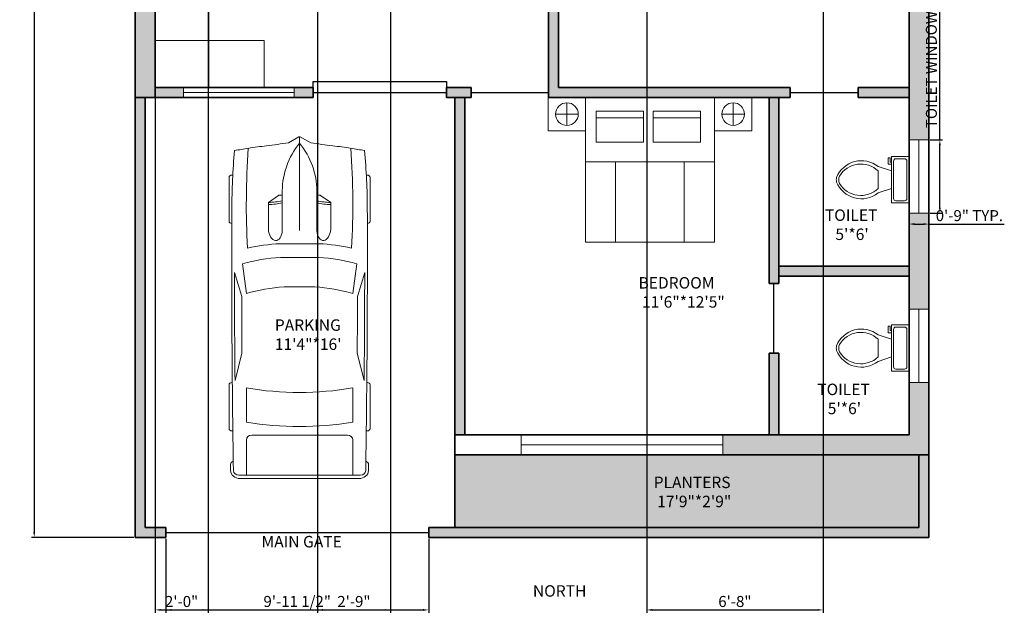
# Model space of a CAD drawing. Units: inches. Extents: x 2066 to 2563, y 1438 to 2142.
# Tile 1 of 3: x 2066 to 2512, y 1438 to 1710. Entities that reach past the tile are written whole.
import ezdxf

# ---------------------------------------------------------------- set-up
doc = ezdxf.new("R2010")
doc.units = ezdxf.units.IN
for name, color, linetype, lineweight in [('A-ANNO-DIMS', 2, 'Continuous', 18), ('A-ANNO-TEXT', 10, 'Continuous', 18), ('A-AREA-IDEN', 10, 'Continuous', 18), ('A-DOOR', 4, 'Continuous', 25), ('A-FLOR-FIXT', 8, 'Continuous', 18), ('A-SITE-VEHS', 8, 'Continuous', 13), ('A-WALL-PATT', 140, 'Continuous', 13), ('BED', 31, 'Continuous', 18), ('FUR', 191, 'Continuous', 18), ('L-PLNT-PATT', 84, 'Continuous', 13), ('WALL', 7, 'Continuous', 35), ('WIND', 210, 'Continuous', 18)]:
    doc.layers.add(name, color=color, linetype=linetype, lineweight=lineweight)
doc.styles.get("Standard").update_dxf_attribs({"font": 'arial.ttf'})
doc.dimstyles.new('ISO-25', dxfattribs={"dimtxt": 5, "dimasz": 2.5, "dimexe": 1.25, "dimexo": 0.625, "dimtad": 1, "dimdec": 0, "dimlunit": 4, "dimtxsty": 'Standard', "dimcen": 2.5, "dimadec": 0, "dimazin": 0, "dimtfac": 1, "dimtdec": 0, "dimtmove": 0, "dimatfit": 3, "dimfxl": 1, "dimarcsym": 0})

# ---------------------------------------------------------------- blocks, each defined once
blk = doc.blocks.new('*U3')
for p, q in [((9.5, -6), (9.5, -2)), ((-10, -8.5), (-8, -8.5)), ((-10, -9.5), (-10, -8.5)), ((-8, -8.5), (-8, -8)), ((-7, -8), (-7, -9.5)), ((-4, -8), (-6, -14)), ((4, -8), (6, -14)), ((-7, -9.5), (-10, -9.5)), ((4, -14), (-4, -14))]:
    blk.add_line(p, q)
blk.add_lwpolyline([(10.5, -8), (10.5, 0), (-10.5, 0), (-10.5, -8)], close=True)
for points in [[(-9.5, -2), (-9.5, -6)], [(8.5, -1), (-8.5, -1)], [(-8.5, -7), (8.5, -7)]]:
    blk.add_lwpolyline(points)
for centre, radius, start, end in [((-8.62, -1.88), 0.884, 81.8699, 188.1301), ((8.62, -1.88), 0.884, 351.8699, 98.1301), ((-8.62, -6.12), 0.884, 171.8699, 278.1301), ((8.62, -6.12), 0.884, 261.8699, 8.1301), ((3.52, -21.58), 12.17, 141.4691, 247.9714), ((4.2, -21.82), 11.33, 136.3677, 238.9468), ((-3.52, -21.58), 12.17, 292.0284, 38.5307), ((-4.2, -21.82), 11.33, 301.053, 43.6321), ((0, -27.88), 4, 245.7318, 294.2682), ((0, -29), 4, 254.8605, 285.1395)]:
    blk.add_arc(centre, radius, start, end)
blk = doc.blocks.new('*U5')
for p, q in [((46.55, 38.89), (22.35, 38.89)), ((136.7, 38.89), (160.9, 38.89)), ((21.1, 37.41), (21.1, 36.83)), ((47.8, 37.39), (47.8, 37.41)), ((87.99, 31.87), (74.76, 35.92)), ((134.31, 35.6), (119.29, 31.78)), ((135.45, 37.07), (135.45, 37.41)), ((162.15, 37.41), (162.15, 36.77)), ((186.47, -33.5), (186.47, 33.5)), ((188.4, -32.76), (188.4, 32.76)), ((70.03, 31.54), (86.41, 29.35)), ((138.42, 29.35), (157.25, 29.35)), ((186.47, 29.35), (167.01, 29.35)), ((164.52, 26.39), (164.52, -26.39)), ((32.27, 11.63), (36.13, 17.17)), ((36.13, 17.17), (50.94, 17.17)), ((32.12, 9.51), (32.12, 11.15)), ((3.27, 6.13), (0.1, 0.41)), ((29.77, 9.51), (51.68, 9.51)), ((58.92, -10.77), (58.92, 10.77)), ((66.55, -10.53), (66.55, 10.53)), ((82.74, 8.5), (82.74, -8.5)), ((186.47, -10.53), (186.47, 10.53)), ((0, 0), (51.68, 0)), ((0.1, -0.41), (3.27, -6.13)), ((29.77, -9.51), (51.68, -9.51)), ((32.12, -9.51), (32.12, -11.15)), ((32.27, -11.63), (36.13, -17.17)), ((36.13, -17.17), (50.94, -17.17)), ((86.41, -29.35), (70.03, -31.54)), ((87.99, -31.87), (74.76, -35.92)), ((134.31, -35.6), (119.29, -31.78)), ((157.25, -29.35), (138.42, -29.35)), ((167.01, -29.35), (186.47, -29.35)), ((21.1, -37.41), (21.1, -36.83)), ((47.8, -37.39), (47.8, -37.41)), ((135.45, -37.07), (135.45, -37.41)), ((162.15, -37.41), (162.15, -36.77)), ((46.55, -38.89), (22.35, -38.89)), ((136.7, -38.89), (160.9, -38.89))]:
    blk.add_line(p, q)
for centre, major_axis, ratio, start_param, end_param in [((22.35, 37.41), (0, -1.48), 0.842304, 3.141593, 4.712389), ((46.55, 37.41), (0, 1.48), 0.842304, -1.570796, 0), ((136.7, 37.41), (0, -1.48), 0.842304, 3.141593, 4.712389), ((160.9, 37.41), (0, 1.48), 0.842304, -1.570796, 0), ((180.63, 35.84), (0, 2.22), 0.842304, -0.013017, 1.249894), ((64.48, -10556.36), (0, 10595.31), 0.842304, -0.013397, -0.013017), ((266.03, -27.52), (0, 313.31), 0.842304, 1.367076, 1.39176), ((41.19, -490.86), (0, 528.23), 0.842304, 0.00281, 0.075598), ((64.48, -10555.62), (0, 10593.03), 0.842304, -0.013397, 0.002797), ((64.48, -10555.62), (0, -10591.55), 0.842304, 3.133765, 3.140441), ((183.98, 33.5), (0, -2.96), 0.842304, 1.570796, 3.128196), ((183.98, 32.76), (0, -5.25), 0.842304, 1.570796, 3.128196), ((259.18, -27.52), (0, -305.3), 0.842304, 4.528606, 4.561838), ((37.47, -593.96), (0, -623.33), 0.842304, 3.096046, 3.200911), ((134.4, 5.39), (0, -89.78), 0.842304, 4.449482, 4.652344), ((135.29, 5.39), (0, 81.77), 0.842304, 1.245306, 1.50788), ((149.6, 2.8), (0, -79.58), 0.842304, 4.372215, 4.640744), ((95.79, -3666.35), (0, -3698.24), 0.842304, 3.134049, 3.144098), ((17.08, 0), (0, 147.02), 0.842304, 4.511394, 4.913384), ((35.91, 0), (0, 147.02), 0.842304, 4.511394, 4.913384), ((167.01, 26.39), (0, 2.96), 0.842304, 0, 1.570796), ((-204.49, 52.4), (0, -250.96), 0.842304, 1.385369, 1.434372), ((13.04, 17.01), (0, 27.42), 0.842304, 4.435146, 4.718221), ((14.2, 17.01), (0, 27.42), 0.842304, 4.435146, 4.718221), ((50.79, 13.34), (6.34, -0.36), 0.603834, -1.395552, 1.581315), ((32.75, 11.15), (0, 0.74), 0.842304, 0.879714, 1.570796), ((29.77, -46.66), (0, 56.17), 0.842304, 0, 0.590319), ((0.62, 0), (0, -0.74), 0.842304, 4.131459, 5.293319), ((29.77, 46.66), (0, 56.17), 0.842304, 2.551274, 3.141593), ((-204.49, -52.4), (0, 250.96), 0.842304, -1.434372, -1.385369), ((13.04, -17.01), (0, -27.42), 0.842304, 1.564964, 1.848039), ((14.2, -17.01), (0, -27.42), 0.842304, 1.564964, 1.848039), ((134.4, -5.39), (0, -89.78), 0.842304, -1.510751, -1.307889), ((135.29, -5.39), (0, -81.77), 0.842304, -1.50788, -1.245306), ((149.6, -2.8), (0, -79.58), 0.842304, -1.499151, -1.230623), ((32.75, -11.15), (0, -0.74), 0.842304, 4.712389, 5.403472), ((259.18, 27.52), (0, 305.3), 0.842304, 1.721348, 1.754579), ((167.01, -26.39), (0, -2.96), 0.842304, 4.712389, 6.283185), ((266.03, 27.52), (0, 313.31), 0.842304, 1.749832, 1.774517), ((37.47, 593.96), (0, -623.33), 0.842304, -0.059319, 0.045547), ((95.79, 3666.35), (0, -3698.24), 0.842304, -0.002505, 0.007544), ((41.19, 490.86), (0, -528.23), 0.842304, -0.075598, -0.00281), ((22.35, -37.41), (0, 1.48), 0.842304, 1.570796, 3.141593), ((64.48, 10555.62), (0, 10593.03), 0.842304, 3.138796, 3.15499), ((46.55, -37.41), (0, -1.48), 0.842304, 0, 1.570796), ((64.48, 10555.62), (0, -10591.55), 0.842304, 0.001152, 0.007828), ((136.7, -37.41), (0, -1.48), 0.842304, -1.570796, 0), ((160.9, -37.41), (0, 1.48), 0.842304, 3.141593, 4.712389), ((180.63, -35.84), (0, -2.22), 0.842304, -1.249894, 0.013017), ((64.48, 10556.36), (0, 10595.31), 0.842304, 3.15461, 3.15499), ((183.98, -33.5), (0, 2.96), 0.842304, 3.15499, 4.712389), ((183.98, -32.76), (0, -5.25), 0.842304, 0.013397, 1.570796)]:
    blk.add_ellipse(centre, major_axis=major_axis, ratio=ratio, start_param=start_param, end_param=end_param)
at = {"extrusion": (0, 0, -1)}
blk.add_ellipse((50.79, -13.34), major_axis=(6.34, 0.36), ratio=0.603834, start_param=-1.395552, end_param=1.581315, dxfattribs=at)
blk = doc.blocks.new('*D9')
at = {"layer": 'A-ANNO-DIMS', "color": 0, "lineweight": -2, "transparency": 16777216}
for p, q in [((2117.45, 2051.04), (2070.96, 2051.04)), ((2072.21, 2048.54), (2072.21, 1477.54)), ((2117.45, 1475.04), (2070.96, 1475.04))]:
    blk.add_line(p, q, dxfattribs=at)
at = {"layer": 'A-ANNO-DIMS', "color": 0, "lineweight": 100, "transparency": 16777216}
for points in [[(2071.79, 2048.54), (2072.63, 2048.54), (2072.21, 2051.04)], [(2071.79, 1477.54), (2072.63, 1477.54), (2072.21, 1475.04)]]:
    blk.add_solid(points, dxfattribs=at)
at = {"layer": 'Defpoints', "color": 0, "lineweight": 100, "transparency": 16777216}
for p in [(2118.07, 2051.04), (2072.21, 1475.04), (2118.07, 1475.04)]:
    blk.add_point(p, dxfattribs=at)
at = {"layer": 'A-ANNO-DIMS', "color": 0, "transparency": 16777216, "insert": (2069.03, 1763.04), "char_height": 5, "attachment_point": 5, "rotation": 90}
blk.add_mtext("48'", dxfattribs=at)
blk = doc.blocks.new('BED-DOUBLE-WITH-NIGHTSTANDS')
for p, q in [((8.49, 52.9), (8.49, 63.16)), ((83.88, 52.9), (83.88, 63.16)), ((3.36, 58.03), (13.62, 58.03)), ((21.71, 56.35), (43.18, 56.35)), ((47.59, 56.35), (69.05, 56.35)), ((78.75, 58.03), (89.01, 58.03)), ((16.98, 36.37), (75.39, 36.37)), ((30.54, 36.37), (30.54, 0)), ((61.6, 36.37), (61.6, 0))]:
    blk.add_line(p, q)
for points in [[(0, 65.59), (16.98, 65.59), (16.98, 50.47), (0, 50.47)], [(16.98, 65.59), (75.39, 65.59), (75.39, 0), (16.98, 0)], [(75.39, 65.59), (92.37, 65.59), (92.37, 50.47), (75.39, 50.47)], [(21.71, 59.42), (43.18, 59.42), (43.18, 45.29), (21.71, 45.29)], [(47.59, 59.42), (69.05, 59.42), (69.05, 45.29), (47.59, 45.29)]]:
    blk.add_lwpolyline(points, close=True)
for centre in [(8.49, 58.03), (83.88, 58.03)]:
    blk.add_circle(centre, 5.13)
blk = doc.blocks.new('WIN-33IN')
blk.add_line((4.5, 0), (4.5, 33.26))
blk.add_lwpolyline([(0, 0), (9, 0), (9, 33.26), (0, 33.26)], close=True)
blk = doc.blocks.new('*D22')
at = {"layer": 'A-ANNO-DIMS', "color": 0, "lineweight": -2, "transparency": 16777216}
for p, q in [((2483.06, 1655.36), (2483.06, 1760.34)), ((2478.7, 1655.36), (2484.31, 1655.36)), ((2483.06, 1624.6), (2483.06, 1652.86)), ((2478.7, 1622.1), (2484.31, 1622.1))]:
    blk.add_line(p, q, dxfattribs=at)
at = {"layer": 'A-ANNO-DIMS', "color": 0, "lineweight": 100, "transparency": 16777216}
for points in [[(2482.64, 1652.86), (2483.48, 1652.86), (2483.06, 1655.36)], [(2482.64, 1624.6), (2483.48, 1624.6), (2483.06, 1622.1)]]:
    blk.add_solid(points, dxfattribs=at)
at = {"layer": 'Defpoints', "color": 0, "lineweight": 100, "transparency": 16777216}
for p in [(2478.07, 1655.36), (2483.06, 1655.36), (2478.07, 1622.1)]:
    blk.add_point(p, dxfattribs=at)
at = {"layer": 'A-ANNO-DIMS', "color": 0, "transparency": 16777216, "insert": (2479.85, 1709.1), "char_height": 5, "attachment_point": 5, "rotation": 90}
blk.add_mtext('TOILET WINDOW 2\'-9 1/2" TYP.', dxfattribs=at)
blk = doc.blocks.new('*D23')
at = {"layer": 'A-ANNO-DIMS', "color": 0, "lineweight": -2, "transparency": 16777216}
for p, q in [((2469.07, 1621.48), (2469.07, 1615.86)), ((2478.07, 1621.48), (2478.07, 1615.86)), ((2471.57, 1617.11), (2475.57, 1617.11)), ((2478.07, 1617.11), (2512.3, 1617.11))]:
    blk.add_line(p, q, dxfattribs=at)
at = {"layer": 'A-ANNO-DIMS', "color": 0, "lineweight": 100, "transparency": 16777216}
for points in [[(2471.57, 1617.53), (2471.57, 1616.7), (2469.07, 1617.11)], [(2475.57, 1617.53), (2475.57, 1616.7), (2478.07, 1617.11)]]:
    blk.add_solid(points, dxfattribs=at)
at = {"layer": 'Defpoints', "color": 0, "lineweight": 100, "transparency": 16777216}
for p in [(2469.07, 1622.1), (2478.07, 1622.1), (2478.07, 1617.11)]:
    blk.add_point(p, dxfattribs=at)
at = {"layer": 'A-ANNO-DIMS', "color": 0, "transparency": 16777216, "insert": (2496.44, 1620.29), "char_height": 5, "attachment_point": 5}
blk.add_mtext('0\'-9" TYP.', dxfattribs=at)
blk = doc.blocks.new('*D28')
at = {"layer": 'A-ANNO-DIMS', "color": 0, "lineweight": -2, "transparency": 16777216}
for p, q in [((2131.87, 1474.42), (2131.87, 1440.89)), ((2251.16, 1474.42), (2251.16, 1440.89)), ((2134.37, 1442.14), (2248.66, 1442.14))]:
    blk.add_line(p, q, dxfattribs=at)
at = {"layer": 'A-ANNO-DIMS', "color": 0, "lineweight": 100, "transparency": 16777216}
for points in [[(2134.37, 1442.56), (2134.37, 1441.73), (2131.87, 1442.14)], [(2248.66, 1442.56), (2248.66, 1441.73), (2251.16, 1442.14)]]:
    blk.add_solid(points, dxfattribs=at)
at = {"layer": 'Defpoints', "color": 0, "lineweight": 100, "transparency": 16777216}
for p in [(2131.87, 1475.04), (2251.16, 1475.04), (2251.16, 1442.14)]:
    blk.add_point(p, dxfattribs=at)
at = {"layer": 'A-ANNO-DIMS', "color": 0, "transparency": 16777216, "insert": (2191.52, 1445.35), "char_height": 5, "attachment_point": 5}
blk.add_mtext('9\'-11 1/2"', dxfattribs=at)
blk = doc.blocks.new('*D29')
at = {"layer": 'A-ANNO-DIMS', "color": 0, "lineweight": -2, "transparency": 16777216}
for p, q in [((2350.07, 1867.92), (2350.07, 1440.89)), ((2430.07, 1867.92), (2430.07, 1440.89)), ((2352.57, 1442.14), (2427.57, 1442.14))]:
    blk.add_line(p, q, dxfattribs=at)
at = {"layer": 'A-ANNO-DIMS', "color": 0, "lineweight": 100, "transparency": 16777216}
for points in [[(2352.57, 1442.56), (2352.57, 1441.73), (2350.07, 1442.14)], [(2427.57, 1442.56), (2427.57, 1441.73), (2430.07, 1442.14)]]:
    blk.add_solid(points, dxfattribs=at)
at = {"layer": 'Defpoints', "color": 0, "lineweight": 100, "transparency": 16777216}
for p in [(2350.07, 1868.54), (2430.07, 1868.54), (2430.07, 1442.14)]:
    blk.add_point(p, dxfattribs=at)
at = {"layer": 'A-ANNO-DIMS', "color": 0, "transparency": 16777216, "insert": (2390.07, 1445.32), "char_height": 5, "attachment_point": 5}
blk.add_mtext('6\'-8"', dxfattribs=at)
blk = doc.blocks.new('*D30')
at = {"layer": 'A-ANNO-DIMS', "color": 0, "lineweight": -2, "transparency": 16777216}
for p, q in [((2127.07, 1883.82), (2127.07, 1440.89)), ((2151.07, 1883.82), (2151.07, 1440.89)), ((2129.57, 1442.14), (2148.57, 1442.14))]:
    blk.add_line(p, q, dxfattribs=at)
at = {"layer": 'A-ANNO-DIMS', "color": 0, "lineweight": 100, "transparency": 16777216}
for points in [[(2129.57, 1442.56), (2129.57, 1441.73), (2127.07, 1442.14)], [(2148.57, 1442.56), (2148.57, 1441.73), (2151.07, 1442.14)]]:
    blk.add_solid(points, dxfattribs=at)
at = {"layer": 'Defpoints', "color": 0, "lineweight": 100, "transparency": 16777216}
for p in [(2127.07, 1884.45), (2151.07, 1884.45), (2151.07, 1442.14)]:
    blk.add_point(p, dxfattribs=at)
at = {"layer": 'A-ANNO-DIMS', "color": 0, "transparency": 16777216, "insert": (2139.07, 1445.32), "char_height": 5, "attachment_point": 5}
blk.add_mtext('2\'-0"', dxfattribs=at)
blk = doc.blocks.new('*D34')
at = {"layer": 'A-ANNO-DIMS', "color": 0, "lineweight": -2, "transparency": 16777216}
for p, q in [((2200.67, 1887.07), (2200.67, 1440.89)), ((2233.8, 1887.07), (2233.8, 1440.89)), ((2203.17, 1442.14), (2231.3, 1442.14))]:
    blk.add_line(p, q, dxfattribs=at)
at = {"layer": 'A-ANNO-DIMS', "color": 0, "lineweight": 100, "transparency": 16777216}
for points in [[(2203.17, 1442.56), (2203.17, 1441.73), (2200.67, 1442.14)], [(2231.3, 1442.56), (2231.3, 1441.73), (2233.8, 1442.14)]]:
    blk.add_solid(points, dxfattribs=at)
at = {"layer": 'Defpoints', "color": 0, "lineweight": 100, "transparency": 16777216}
for p in [(2200.67, 1887.69), (2233.8, 1887.69), (2233.8, 1442.14)]:
    blk.add_point(p, dxfattribs=at)
at = {"layer": 'A-ANNO-DIMS', "color": 0, "transparency": 16777216, "insert": (2217.24, 1445.32), "char_height": 5, "attachment_point": 5}
blk.add_mtext('2\'-9"', dxfattribs=at)

msp = doc.modelspace()

# ---------------------------------------------------------------- hatches: boundary and pattern name
at = {"layer": 'A-WALL-PATT'}
h = msp.add_hatch(color=256, dxfattribs=at)
h.dxf.hatch_style = 1
h.paths.add_polyline_path([(2210.43, 2051.04), (2194.82, 2051.04), (2194.82, 2042.04), (2210.43, 2042.04)])
h.paths.add_polyline_path([(2265.69, 2051.04), (2243.73, 2051.04), (2243.73, 2042.04), (2265.69, 2042.04)])
h.paths.add_polyline_path([(2478.07, 2051.04), (2288.73, 2051.04), (2288.73, 2042.04), (2288.96, 2042.04), (2469.07, 2042.04), (2469.07, 2021.26), (2478.07, 2021.26)])
h.paths.add_polyline_path([(2127.07, 2042.04), (2134.17, 2042.04), (2134.17, 2051.04), (2118.07, 2051.04), (2118.07, 1957.11), (2127.07, 1957.11), (2127.07, 1977.54)])
h.paths.add_polyline_path([(2201.01, 1982.04), (2127.07, 1982.04), (2127.07, 1977.54), (2201.01, 1977.54)])
h.paths.add_polyline_path([(2247.07, 1982.04), (2241.78, 1982.04), (2241.78, 1977.54), (2247.07, 1977.54)])
h.paths.add_polyline_path([(2251.57, 2042.04), (2247.07, 2042.04), (2247.07, 1954.54), (2310.07, 1954.54), (2310.07, 1964.11), (2305.57, 1964.11), (2305.57, 1959.04), (2251.57, 1959.04)])
h.paths.add_polyline_path([(2310.07, 2042.04), (2305.57, 2042.04), (2305.57, 2000.54), (2310.07, 2000.54)], flags=17)
h.paths.add_polyline_path([(2478.07, 1938.37), (2469.07, 1938.37), (2469.07, 1846.24), (2478.07, 1846.24)])
h.paths.add_polyline_path([(2469.07, 1910.04), (2384.89, 1910.04), (2370.05, 1910.04), (2318.28, 1910.04), (2310.07, 1910.04), (2310.07, 1919.07), (2305.57, 1919.07), (2305.57, 1910.04), (2305.57, 1905.54), (2310.07, 1905.54), (2318.28, 1905.54), (2370.05, 1905.54), (2469.07, 1905.54)])
h.paths.add_polyline_path([(2469.07, 1868.54), (2408.15, 1868.54), (2408.15, 1858.69), (2412.15, 1858.69), (2412.15, 1864.54), (2469.07, 1864.54)])
h.paths.add_polyline_path([(2469.07, 1827.54), (2359.25, 1827.54), (2359.25, 1823.04), (2469.07, 1823.04)])
h.paths.add_polyline_path([(2314.44, 1827.54), (2310.07, 1827.54), (2305.57, 1827.54), (2305.57, 1743.86), (2305.57, 1723.24), (2305.57, 1679.04), (2305.57, 1674.54), (2322.38, 1674.54), (2380.79, 1674.54), (2397.77, 1674.54), (2415.18, 1674.54), (2415.18, 1679.04), (2310.07, 1679.04), (2310.07, 1823.04), (2314.44, 1823.04)])
h.paths.add_polyline_path([(2478.07, 1763.36), (2469.07, 1763.36), (2469.07, 1655.36), (2478.07, 1655.36)])
h.paths.add_polyline_path([(2469.07, 1679.04), (2446.03, 1679.04), (2446.03, 1674.54), (2469.07, 1674.54)])
h.paths.add_polyline_path([(2410.07, 1670.54), (2410.07, 1674.54), (2405.57, 1674.54), (2405.57, 1670.54), (2405.57, 1590.09), (2410.07, 1590.09), (2410.07, 1593.54)])
h.paths.add_polyline_path([(2469.07, 1598.04), (2410.07, 1598.04), (2410.07, 1593.54), (2469.07, 1593.54)])
h.paths.add_polyline_path([(2478.07, 1622.1), (2469.07, 1622.1), (2469.07, 1578.59), (2478.07, 1578.59)])
h.paths.add_polyline_path([(2478.07, 1545.33), (2469.07, 1545.33), (2469.07, 1521.54), (2384.6, 1521.54), (2384.6, 1512.54), (2473.57, 1512.54), (2478.07, 1512.54)])
h.paths.add_polyline_path([(2410.07, 1558.62), (2405.57, 1558.62), (2405.57, 1521.54), (2410.07, 1521.54)])
h.paths.add_polyline_path([(2478.07, 1512.54), (2473.57, 1512.54), (2473.57, 1479.54), (2263.07, 1479.54), (2251.16, 1479.54), (2251.16, 1475.04), (2478.07, 1475.04)])
h.paths.add_polyline_path([(2122.57, 1674.54), (2118.07, 1674.54), (2118.07, 1475.04), (2131.87, 1475.04), (2131.87, 1479.54), (2122.57, 1479.54)])
h.paths.add_polyline_path([(2267.57, 1674.54), (2263.07, 1674.54), (2263.07, 1521.54), (2267.57, 1521.54)])
h.paths.add_polyline_path([(2270.46, 1679.04), (2259.18, 1679.04), (2259.18, 1674.54), (2263.07, 1674.54), (2270.46, 1674.54)])
h.paths.add_polyline_path([(2198.77, 1679.04), (2190.12, 1679.04), (2190.12, 1674.54), (2198.77, 1674.54)])
h.paths.add_polyline_path([(2139.93, 1679.04), (2127.07, 1679.04), (2127.07, 1674.54), (2139.93, 1674.54)])
h.paths.add_polyline_path([(2127.07, 1700.37), (2127.07, 1732.8), (2118.07, 1732.8), (2118.07, 1674.54), (2122.57, 1674.54), (2127.07, 1674.54), (2127.07, 1679.04)])
h.paths.add_polyline_path([(2127.07, 1879.08), (2118.07, 1879.08), (2118.07, 1810.83), (2127.07, 1810.83), (2127.07, 1823.04)])
h.paths.add_polyline_path([(2200.14, 1827.54), (2127.07, 1827.54), (2127.07, 1823.04), (2151.5, 1823.04), (2176.6, 1823.04), (2200.14, 1823.04)])
at = {"layer": 'L-PLNT-PATT'}
h = msp.add_hatch(color=256, dxfattribs=at)
h.dxf.hatch_style = 1
h.paths.add_polyline_path([(2473.57, 1512.54), (2267.57, 1512.54), (2263.07, 1512.54), (2263.07, 1479.54), (2473.57, 1479.54)])

# ---------------------------------------------------------------- linework, layer by layer
at = {"layer": 'A-DOOR'}
for p, q in [((2198.77, 1676.79), (2198.77, 1681.73)), ((2198.77, 1681.73), (2259.18, 1681.73)), ((2259.18, 1681.73), (2259.18, 1679.04)), ((2198.77, 1676.79), (2259.18, 1676.79)), ((2270.46, 1676.79), (2305.57, 1676.79)), ((2415.18, 1676.79), (2446.03, 1676.79)), ((2407.82, 1558.62), (2407.82, 1590.09)), ((2131.87, 1477.29), (2251.16, 1477.29))]:
    msp.add_line(p, q, dxfattribs=at)
at = {"layer": 'FUR'}
for points in [[(2127.07, 1823.04), (2151.5, 1823.04), (2151.5, 1679.04), (2127.07, 1679.04)], [(2176.6, 1700.37), (2127.07, 1700.37), (2127.07, 1679.04), (2176.6, 1679.04)]]:
    msp.add_lwpolyline(points, close=True, dxfattribs=at)
at = {"layer": 'WALL'}
for p, q in [((2118.07, 1475.04), (2118.07, 2051.04)), ((2478.07, 2051.04), (2478.07, 1475.04)), ((2127.07, 1674.54), (2127.07, 2042.04)), ((2469.07, 2042.04), (2469.07, 1521.54)), ((2127.07, 1823.04), (2127.07, 1679.04)), ((2310.07, 1823.04), (2310.07, 1679.04)), ((2310.07, 1679.04), (2310.07, 1823.04)), ((2305.57, 1743.86), (2305.57, 1679.04)), ((2127.07, 1679.04), (2198.77, 1679.04)), ((2259.18, 1679.04), (2270.46, 1679.04)), ((2270.46, 1674.54), (2270.46, 1679.04)), ((2305.57, 1679.04), (2305.57, 1674.54)), ((2310.07, 1679.04), (2415.18, 1679.04)), ((2446.03, 1679.04), (2469.07, 1679.04)), ((2127.07, 1674.54), (2118.07, 1674.54)), ((2122.57, 1674.54), (2122.57, 1479.54)), ((2127.07, 1674.54), (2198.77, 1674.54)), ((2127.07, 1674.54), (2198.77, 1674.54)), ((2259.18, 1674.54), (2263.07, 1674.54)), ((2259.18, 1674.54), (2270.46, 1674.54)), ((2263.07, 1674.54), (2263.07, 1484.04)), ((2267.57, 1674.54), (2267.57, 1521.54)), ((2305.57, 1674.54), (2310.07, 1674.54)), ((2310.07, 1674.54), (2415.18, 1674.54)), ((2405.57, 1670.54), (2405.57, 1674.54)), ((2410.07, 1670.54), (2410.07, 1674.54)), ((2446.03, 1674.54), (2469.07, 1674.54)), ((2405.57, 1590.09), (2405.57, 1670.54)), ((2410.07, 1590.09), (2410.07, 1670.54)), ((2410.07, 1598.04), (2469.07, 1598.04)), ((2410.07, 1593.54), (2469.07, 1593.54)), ((2410.07, 1590.09), (2410.07, 1593.54)), ((2405.57, 1590.09), (2410.07, 1590.09)), ((2405.57, 1521.54), (2405.57, 1558.62)), ((2405.57, 1558.62), (2410.07, 1558.62)), ((2410.07, 1521.54), (2410.07, 1558.62)), ((2410.07, 1521.54), (2410.07, 1558.62)), ((2267.57, 1521.54), (2263.07, 1521.54)), ((2263.07, 1521.54), (2267.57, 1521.54)), ((2267.57, 1521.54), (2469.07, 1521.54)), ((2267.57, 1521.54), (2405.57, 1521.54)), ((2263.07, 1479.54), (2263.07, 1512.54)), ((2267.57, 1512.54), (2263.07, 1512.54)), ((2263.07, 1512.54), (2267.57, 1512.54)), ((2267.57, 1512.54), (2473.57, 1512.54)), ((2473.57, 1512.54), (2473.57, 1479.54)), ((2473.57, 1512.54), (2478.07, 1512.54)), ((2263.07, 1484.04), (2263.07, 1479.54)), ((2122.57, 1479.54), (2131.87, 1479.54)), ((2131.87, 1479.54), (2131.87, 1475.04)), ((2263.07, 1479.54), (2251.16, 1479.54)), ((2251.16, 1479.54), (2251.16, 1475.04)), ((2263.07, 1479.54), (2473.57, 1479.54)), ((2118.07, 1475.04), (2131.87, 1475.04)), ((2478.07, 1475.04), (2251.16, 1475.04))]:
    msp.add_line(p, q, dxfattribs=at)
for points in [[(2198.77, 1679.04), (2198.77, 1674.54)], [(2259.18, 1674.54), (2259.18, 1679.04)], [(2415.18, 1679.04), (2415.18, 1674.54)], [(2446.03, 1674.54), (2446.03, 1679.04)]]:
    msp.add_lwpolyline(points, dxfattribs=at)
at = {"layer": 'WIND'}
for p, q in [((2139.93, 1676.79), (2190.12, 1676.79)), ((2293.17, 1517.04), (2384.6, 1517.04))]:
    msp.add_line(p, q, dxfattribs=at)
for points in [[(2190.12, 1679.04), (2139.93, 1679.04), (2139.93, 1674.54), (2190.12, 1674.54)], [(2293.17, 1521.54), (2384.6, 1521.54), (2384.6, 1512.54), (2293.17, 1512.54)]]:
    msp.add_lwpolyline(points, close=True, dxfattribs=at)

# ---------------------------------------------------------------- block references
at = {"layer": 'A-FLOR-FIXT', "rotation": 270}
for p in [(2469.07, 1637.21), (2469.07, 1560.86)]:
    msp.add_blockref('*U3', p, dxfattribs=at)
at = {"layer": 'A-SITE-VEHS', "xscale": 0.8225747121648183, "yscale": 0.8225747121648183, "zscale": 0.8225747121648183, "rotation": 270}
msp.add_blockref('*U5', (2192.59, 1656.68), dxfattribs=at)
at = {"layer": 'BED'}
msp.add_blockref('BED-DOUBLE-WITH-NIGHTSTANDS', (2305.4, 1608.95), dxfattribs=at)
at = {"layer": 'WIND'}
for p in [(2469.07, 1622.1), (2469.07, 1545.33)]:
    msp.add_blockref('WIN-33IN', p, dxfattribs=at)

# ---------------------------------------------------------------- texts
at = {"layer": 'A-ANNO-TEXT', "char_height": 5.193, "attachment_point": 1}
for s, insert in [('MAIN GATE', (2175.32, 1475.69)), ('NORTH', (2298.45, 1453.35))]:
    msp.add_mtext_dynamic_manual_height_columns(s, width=129.7814, gutter_width=25.96, heights=[0], dxfattribs=dict(at, insert=insert))
at = {"layer": 'A-AREA-IDEN', "attachment_point": 1}
for s, insert, char_height in [("TOILET\\P   5'*6'", (2430.91, 1623.74), 5.193), ('BEDROOM\\P 11\'6"*12\'5"', (2346.35, 1593.06), 5.1929), ('PARKING\\P11\'4"*16\'', (2181.37, 1573.9), 5.193), ("TOILET\\P   5'*6'", (2427.45, 1544.75), 5.193), ('PLANTERS\\P 17\'9"*2\'9"', (2353.23, 1502.58), 5.1929)]:
    msp.add_mtext_dynamic_manual_height_columns(s, width=129.7814, gutter_width=25.96, heights=[0], dxfattribs=dict(at, insert=insert, char_height=char_height))

# ---------------------------------------------------------------- dimensions: what is measured, and where the dimension line sits
at = {"layer": 'A-ANNO-DIMS'}
dim = msp.add_linear_dim(base=(2072.21, 1475.04), p1=(2118.07, 2051.04), p2=(2118.07, 1475.04), angle=90, dimstyle='ISO-25', override={"dimclrd": 0, "dimclre": 0, "dimclrt": 0}, dxfattribs=at)
dim.commit()
dim.dimension.update_dxf_attribs({"geometry": '*D9', "text_midpoint": (2069.03, 1763.04)})
for base, p1, p2, picture, middle in [((2233.8, 1442.14), (2200.67, 1887.69), (2233.8, 1887.69), '*D34', (2217.24, 1445.32)), ((2151.07, 1442.14), (2127.07, 1884.45), (2151.07, 1884.45), '*D30', (2139.07, 1445.32)), ((2430.07, 1442.14), (2350.07, 1868.54), (2430.07, 1868.54), '*D29', (2390.07, 1445.32)), ((2251.16, 1442.14), (2131.87, 1475.04), (2251.16, 1475.04), '*D28', (2191.52, 1445.35))]:
    dim = msp.add_linear_dim(base=base, p1=p1, p2=p2, dimstyle='ISO-25', override={"dimdec": 1, "dimlfac": 1, "dimrnd": 0, "dimzin": 1, "dimdsep": 46, "dimlunit": 4, "dimfrac": 2}, dxfattribs=at)
    dim.commit()
    dim.dimension.update_dxf_attribs({"geometry": picture, "text_midpoint": middle})
dim = msp.add_linear_dim(base=(2483.06, 1655.36), p1=(2478.07, 1622.1), p2=(2478.07, 1655.36), angle=90, text='TOILET WINDOW <> TYP.', dimstyle='ISO-25', override={"dimdec": 1, "dimlfac": 1, "dimrnd": 0, "dimzin": 1, "dimdsep": 46, "dimlunit": 4, "dimfrac": 2}, dxfattribs=at)
dim.commit()
dim.dimension.update_dxf_attribs({"geometry": '*D22', "text_midpoint": (2479.85, 1709.1)})
dim = msp.add_linear_dim(base=(2478.07, 1617.11), p1=(2469.07, 1622.1), p2=(2478.07, 1622.1), text='<> TYP.', dimstyle='ISO-25', override={"dimdec": 1, "dimlfac": 1, "dimrnd": 0, "dimzin": 1, "dimdsep": 46, "dimlunit": 4, "dimfrac": 2}, dxfattribs=at)
dim.commit()
dim.dimension.update_dxf_attribs({"geometry": '*D23', "text_midpoint": (2496.44, 1620.29)})

doc.saveas('drawing.dxf')
